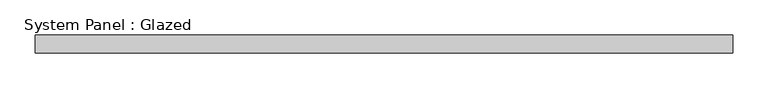
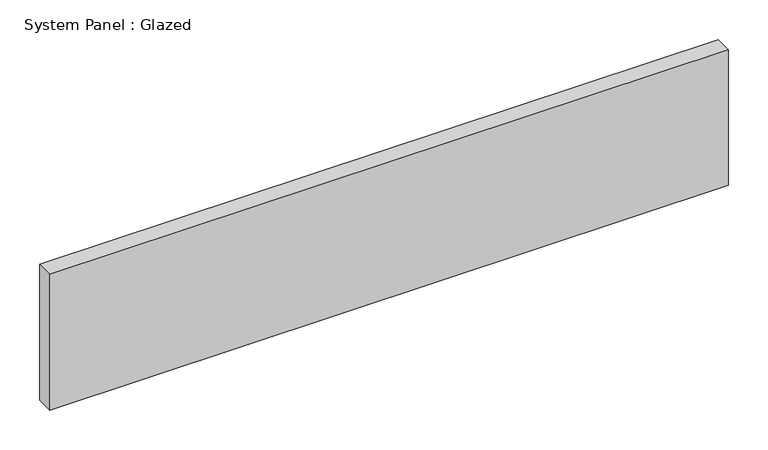
"""IFC4 building model written with IfcOpenShell, lengths in millimetres: plate geometry, System Panel : Glazed."""

from ifc_helpers import new_model, si_unit, origin, origin_with_axes, place, context, project, spatial, polyline, outline, extrude, source, transform, mapped, element, save


def system_panel_glazed_7419534f(model_context):
    return source(origin(), model_context, "Body", "SweptSolid", [
        extrude(outline(polyline([(495.3, 19.05), (-495.3, 19.05), (-495.3, 44.45), (495.3, 44.45), (495.3, 19.05)])), origin_with_axes(), (0.0, 0.0, 1.0), 209.55),
    ])


if __name__ == "__main__":
    model = new_model("IFC4")
    model_context = context("Model", 3, world=origin())
    ifc_project = project(units=[si_unit("LENGTHUNIT", "METRE", prefix="MILLI")], contexts=[model_context])
    site = spatial("IfcSite", under=ifc_project)
    building = spatial("IfcBuilding", under=site)
    placement = place(None, origin())
    system_panel_glazed_shape = system_panel_glazed_7419534f(model_context)
    element("IfcPlate", 1, ObjectType="System Panel : Glazed", at=placement, inside=building, context=model_context, shape_type="MappedRepresentation", body=[
        mapped(system_panel_glazed_shape, transform((0.0, 0.0, 0.0), x_axis=(1.0, 0.0, 0.0), y_axis=(0.0, 1.0, 0.0), z_axis=(0.0, 0.0, 1.0))),
    ])
    save(model, "model.ifc")

# Revit data of these elements
# Type "System Panel : Glazed"
#   Construction Type Id = "GSP4R"
#   Analytic Construction = "1/8 in Pilkington single glazing"
#   Visual Light Transmittance = 0.9
#   Solar Heat Gain Coefficient = 0.86
#   Heat Transfer Coefficient (U) = 1.18115 BTU/(h·ft²·°F)
#   Define Thermal Properties by = 1
# Element 1 (IfcPlate, "System Panel : Glazed")
#   Materials on its faces: "Glass"
# Materials
#   "Glass": class "Glass", colour RGB 0 128 192, transparency 0.75, Description = "Soda Lime Glass", Cost = 0
